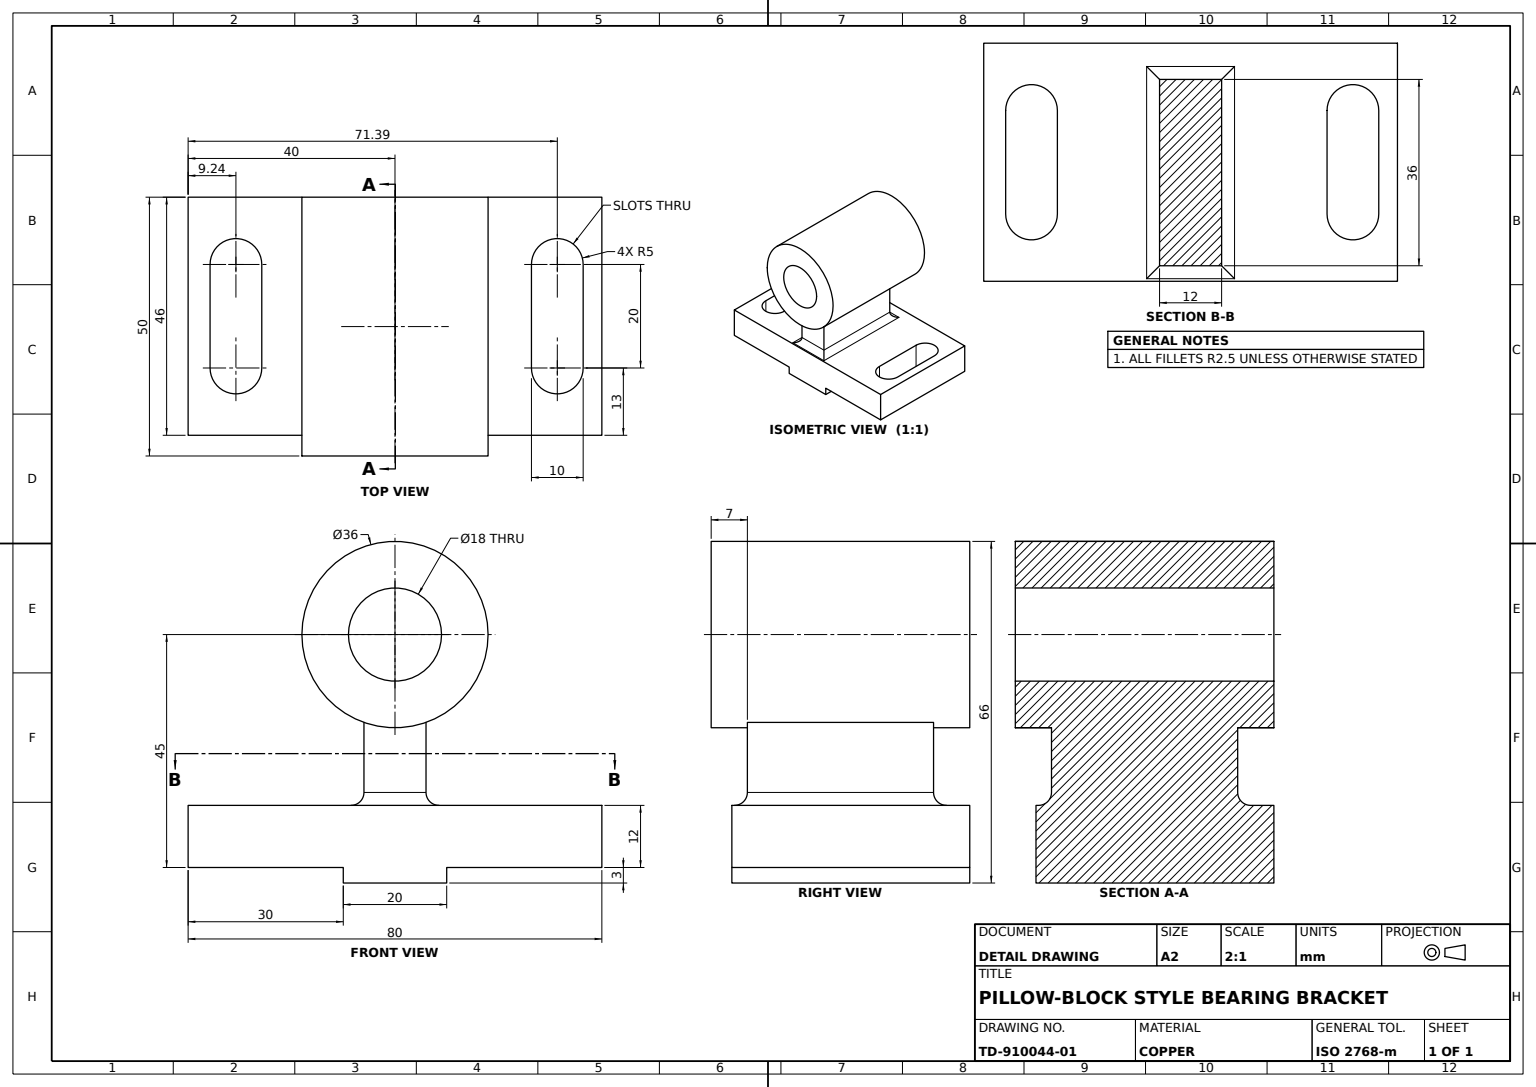
SolidWorks part; units mm, degrees
material "Copper"
ref_plane "Front Plane" through (0, 0, 0) normal (0, 0, 1) x (1, 0, 0)
ref_plane "Top Plane" through (0, 0, 0) normal (0, 1, 0) x (1, 0, 0)
ref_plane "Right Plane" through (0, 0, 0) normal (1, 0, 0) x (0, 0, -1)
sketch "Base Plate Profile" plane through (0, 0, 0) normal (1, 0, 0) x (0, 0, -1)
  line L0 (0, 0) -> (30, 0)
  line L1 (30, 0) -> (30, -3)
  line L2 (30, -3) -> (50, -3)
  line L3 (50, -3) -> (50, 0)
  line L4 (50, 0) -> (80, 0)
  line L5 (80, 0) -> (80, 12)
  line L6 (80, 12) -> (0, 12)
  line L7 (0, 12) -> (0, 0)
  dimension "D1" = 12
  dimension "D2" = 80
  dimension "D3" = 20
  dimension "D4" = 30
  dimension "D5" = 3
extrude "Base Plate" add sketch "Base Plate Profile" along normal blind 46 contours L6 L7 L0 L1 L2 L3 L4 L5
sketch "Hub Profile Ø36-Ø18" plane through (0, 0, 0) normal (-1, 0, 0) x (0, 0, 1)
  line L0 (-50, 0) -> (-80, 0) construction
  circle A0 centre (-40, 45) radius 18
  circle A1 centre (-40, 45) radius 9
  dimension "D1" = 36
  dimension "D2" = 18
  dimension "D3" = 45
  dimension "D4" = 40
extrude "Bearing Hub Ø36 Bore Ø18" add sketch "Hub Profile Ø36-Ø18" against normal blind 50 separate body
sketch "Hub Support Profile" plane through (0, 12, 0) normal (0, 1, 0) x (1, 0, 0)
  line L0 (0, 40) -> (50, 40)
  line L1 (0, 58) -> (0, 22) construction
  line L2 (50, 22) -> (50, 58) construction
  line L4 (43, 34) -> (7, 34)
  line L5 (43, 34) -> (43, 46)
  line L6 (43, 46) -> (7, 46)
  line L7 (7, 34) -> (7, 46)
  line L8 (43, 34) -> (7, 46) construction
  line L9 (43, 46) -> (7, 34) construction
  point P6 (25, 40)
  dimension "D1" = 36
  dimension "D2" = 12
extrude "Hub Support Web" add sketch "Hub Support Profile" along normal up to surface (16.0294 mm away) contours L4 L7 L6 L5
sketch "Mounting Slots Profile" plane through (0, 12, 0) normal (0, 1, 0) x (1, 0, 0)
  line L0 (13, 71.3852) -> (33, 71.3852) construction
  line L1 (13, 76.3852) -> (33, 76.3852)
  line L2 (13, 66.3852) -> (33, 66.3852)
  line L3 (13, 9.2433) -> (33, 9.2433) construction
  line L4 (13, 14.2433) -> (33, 14.2433)
  line L5 (13, 4.2433) -> (33, 4.2433)
  line L6 (0, 80) -> (0, 0) construction
  arc A0 (13, 76.3852) -> (13, 66.3852) centre (13, 71.3852) ccw
  arc A1 (33, 66.3852) -> (33, 76.3852) centre (33, 71.3852) ccw
  arc A2 (13, 14.2433) -> (13, 4.2433) centre (13, 9.2433) ccw
  arc A3 (33, 4.2433) -> (33, 14.2433) centre (33, 9.2433) ccw
  point P2 (23, 71.3852)
  point P7 (23, 9.2433)
  dimension "D1" = 13
  dimension "D2" = 20
  dimension "D3" = 10
  dimension "D4" = 13
  dimension "D5" = 10
  dimension "D6" = 20
  dimension "D7" = 71.3852
  dimension "D8" = 9.2433
extrude "Mounting Slots 2x" cut sketch "Mounting Slots Profile" against normal through all
fillet "Edge Fillets R2.5" radius 2.5 4 edges at (25, 12, -46) (7, 12, -40) (43, 12, -40) (25, 12, -34)
